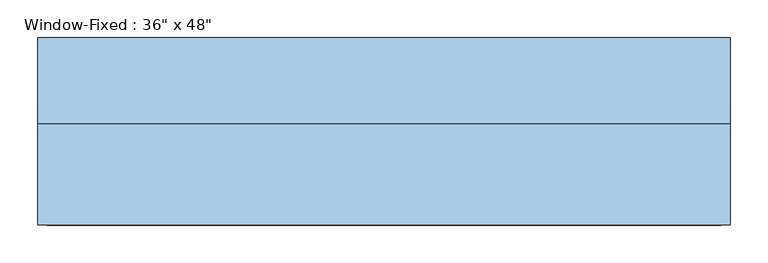
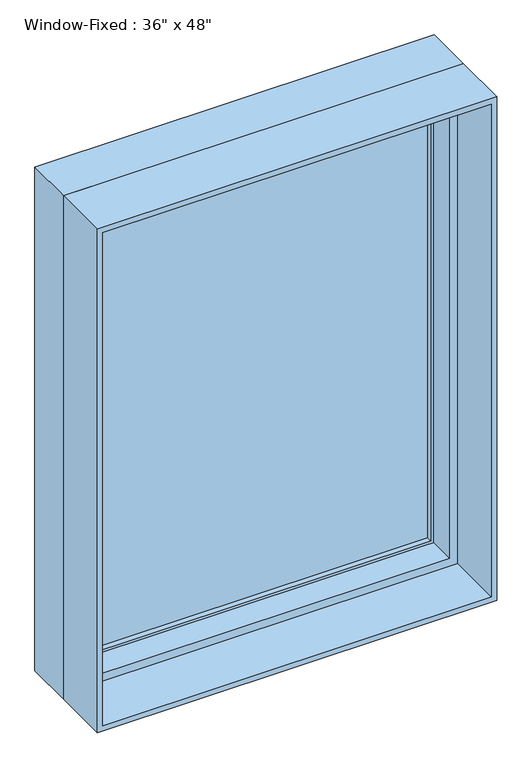
"""IFC4 building model written with IfcOpenShell, lengths in millimetres: window geometry."""

from ifc_helpers import new_model, si_unit, frame, origin, place, context, project, spatial, polyline, outline, extrude, faceted_brep, source, transform, mapped, element, save


def window_2799360a(model_context):
    return source(origin(), model_context, "Body", "SolidModel", [
        extrude(outline(polyline([(419.1, 114.3), (419.1, 107.95), (-419.1, 107.95), (-419.1, 114.3), (419.1, 114.3)])), frame((0.0, 0.0, 952.5), z_axis=(0.0, 0.0, 1.0), x_axis=(1.0, 0.0, 0.0)), (0.0, 0.0, 1.0), 1143.0),
        extrude(outline(polyline([(-419.1, 95.25), (-419.1, 101.6), (419.1, 101.6), (419.1, 95.25), (-419.1, 95.25)])), frame((0.0, 0.0, 952.5), z_axis=(0.0, 0.0, 1.0), x_axis=(1.0, 0.0, 0.0)), (0.0, 0.0, 1.0), 1143.0),
        extrude(outline(polyline([(927.1, 444.5), (2120.9, 444.5), (2120.9, -444.5), (927.1, -444.5), (927.1, 444.5)]), holes=[polyline([(952.5, -419.1), (2095.5, -419.1), (2095.5, 419.1), (952.5, 419.1), (952.5, -419.1)])]), frame((0.0, 82.55, 0.0), z_axis=(0.0, 1.0, 0.0), x_axis=(0.0, 0.0, 1.0)), (0.0, 0.0, 1.0), 44.45),
        extrude(outline(polyline([(2133.6, -457.2), (914.4, -457.2), (914.4, 457.2), (2133.6, 457.2), (2133.6, -457.2)]), holes=[polyline([(2120.9, 444.5), (927.1, 444.5), (927.1, -444.5), (2120.9, -444.5), (2120.9, 444.5)])]), frame((0.0, -114.3, 0.0), z_axis=(0.0, 1.0, 0.0), x_axis=(0.0, 0.0, 1.0)), (0.0, 0.0, 1.0), 133.35),
        faceted_brep([(457.2, 19.05, 2133.6), (457.2, 133.35, 2133.6), (-457.2, 133.35, 2133.6), (-457.2, 19.05, 2133.6), (-457.2, 133.35, 914.4), (-457.2, 19.05, 914.4), (457.2, 133.35, 914.4), (457.2, 19.05, 914.4), (425.45, 19.05, 2101.85), (425.45, 19.05, 946.15), (-425.45, 19.05, 946.15), (-425.45, 19.05, 2101.85), (-444.5, 133.35, 2120.9), (-444.5, 133.35, 927.1), (444.5, 133.35, 927.1), (444.5, 133.35, 2120.9), (425.45, 82.55, 2101.85), (-425.45, 82.55, 2101.85), (444.5, 82.55, 2120.9), (-444.5, 82.55, 2120.9), (-425.45, 82.55, 946.15), (-444.5, 82.55, 927.1), (425.45, 82.55, 946.15), (444.5, 82.55, 927.1)], [[[0, 1, 2, 3]], [[3, 2, 4, 5]], [[5, 4, 6, 7]], [[3, 5, 7, 0], [8, 9, 10, 11]], [[7, 6, 1, 0]], [[1, 6, 4, 2], [12, 13, 14, 15]], [[16, 8, 11, 17]], [[15, 18, 19, 12]], [[17, 11, 10, 20]], [[12, 19, 21, 13]], [[20, 10, 9, 22]], [[13, 21, 23, 14]], [[22, 9, 8, 16]], [[18, 23, 21, 19], [17, 20, 22, 16]], [[14, 23, 18, 15]]]),
    ])


if __name__ == "__main__":
    model = new_model("IFC4")
    model_context = context("Model", 3, world=origin())
    ifc_project = project(units=[si_unit("LENGTHUNIT", "METRE", prefix="MILLI")], contexts=[model_context])
    site = spatial("IfcSite", under=ifc_project)
    building = spatial("IfcBuilding", under=site)
    placement = place(None, origin())
    window_shape = window_2799360a(model_context)
    element("IfcWindow", 1, ObjectType="Window-Fixed : 36\" x 48\"", at=placement, inside=building, context=model_context, shape_type="MappedRepresentation", body=[
        mapped(window_shape, transform((0.0, 0.0, 0.0), x_axis=(1.0, 0.0, 0.0), y_axis=(0.0, 1.0, 0.0), z_axis=(0.0, 0.0, 1.0))),
    ])
    save(model, "model.ifc")

# Revit data of these elements
# Type "Window-Fixed : 36\" x 48\""
#   Type Mark = "22"
#   Fire Rating = "0.5h"
#   Assembly Code = "B2020100"
#   Analytic Construction = "Double glazing - domestic"
#   Window Inset [instance default] = 0' - 0"
#   Wall Thickness [instance default] = 0' - 6"
#   Visual Light Transmittance = 0.81
#   Thermal Resistance (R) = 1.8146 (h·ft²·°F)/BTU
#   Solar Heat Gain Coefficient = 0.76
#   Rough Width = 3' - 0 1/2"
#   Rough Height = 4' - 0 1/2"
#   Interior Wall Closure [instance default] = 0' - 2 1/4"
#   Height = 4' - 0"
#   Heat Transfer Coefficient (U) = 0.5511 BTU/(h·ft²·°F)
#   Frame Extension [instance default] = 0' - 0 1/4"
#   Exterior Wall Closure [instance default] = 0' - 1 1/4"
#   Extension Jamb [instance default] = 0' - 2 1/4"
#   Default Sill Height = 3' - 0"
#   Width = 3' - 0"
#   Muntin Visibility = yes
#   Interior Trim Visibility [instance default] = yes
#   Exterior Trim Visibility [instance default] = yes
#   Extension Jamb Visibility [instance default] = yes
#   Define Thermal Properties by = 1
#   Muntin Pattern = Muntin Pattern_2x2 : Muntin Pattern_2x2
#   Interior Trim Material = Wood - Stained
#   Interior Trim = Trim-Window-Interior-Flat : Picture Frame
#   Interior Frame Material = Wood - Stained
#   Glass Panel Material = Glass
#   Exterior Trim Material = Clad - White
#   Exterior Trim = Trim-Window-Exterior-Flat : with Sill
#   Exterior Frame Material = Clad - White
#   Wall Closure = (empty or 0)
# Element 1 (IfcWindow, "Window-Fixed : 36\" x 48\"")
#   Wall Thickness = 0' - 9"
#   Extension Jamb = 0' - 5 1/4"
#   Materials on its faces: "Wood - Stained", "Glass", "Clad - White"
# Materials
#   "Wood - Stained": class "Wood", colour RGB 173 132 96, transparency 0, Cost = 0
#   "Glass": class "Glass", colour RGB 245 245 243, transparency 1, Description = "Soda Lime Glass", Cost = 0
#   "Clad - White": class "Wood", colour RGB 245 245 243, transparency 0, Cost = 0
